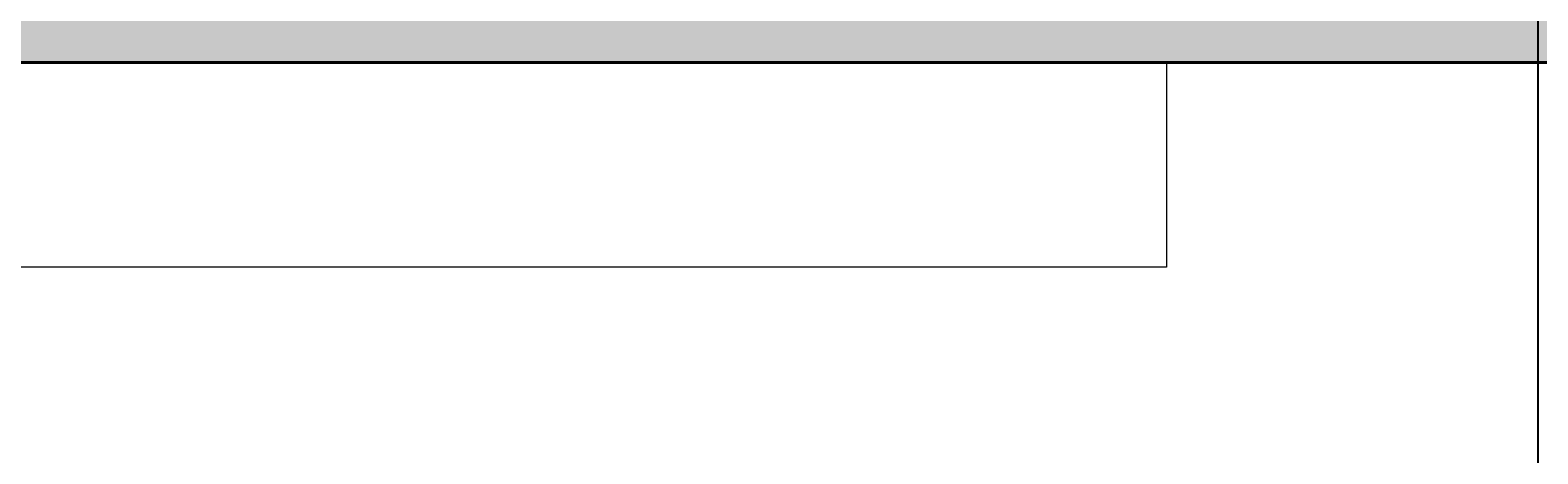
# Model space of a CAD drawing. Units: inches. Extents: x 1998 to 2588, y 1139 to 1977.
# Tile 92 of 134: x 2453 to 2498, y 1465 to 1477. Entities that reach past the tile are written whole.
import ezdxf

# ---------------------------------------------------------------- set-up
doc = ezdxf.new("R2010")
doc.units = ezdxf.units.IN
for name, color, linetype, lineweight in [('A-ANNO-DIMS', 2, 'Continuous', 18), ('A-WALL-PATT', 252, 'Continuous', 13), ('FUR', 21, 'Continuous', 18), ('WALL', 200, 'Continuous', 35)]:
    doc.layers.add(name, color=color, linetype=linetype, lineweight=lineweight)
doc.styles.get("Standard").update_dxf_attribs({"font": 'arial.ttf'})
doc.dimstyles.get("Standard").update_dxf_attribs({"dimtxt": 0.18, "dimasz": 0.18, "dimexe": 0.18, "dimexo": 0.0625, "dimgap": 0.09, "dimtad": 0, "dimtih": 1, "dimtoh": 1, "dimdec": 4, "dimzin": 0, "dimdsep": 46, "dimtxsty": 'Standard', "dimcen": 0.09, "dimadec": 0, "dimazin": 0, "dimtfac": 1, "dimtdec": 4, "dimtofl": 0, "dimtmove": 0, "dimatfit": 3, "dimfxl": 1, "dimtolj": 1, "dimtzin": 0, "dimarcsym": 0})

# ---------------------------------------------------------------- blocks, each defined once
blk = doc.blocks.new('CONSOLE-WALL')
blk.add_lwpolyline([(0, 6.123), (71.98, 6.123), (71.98, 0), (0, 0)], close=True)
blk = doc.blocks.new('*D23')
at = {"layer": 'A-ANNO-DIMS', "color": 0, "lineweight": -2, "transparency": 16777216}
for p, q in [((2549.179, 1476.17), (2549.179, 1138.602)), ((2059.473, 1413.17), (2059.473, 1138.602)), ((2059.653, 1138.782), (2303.928, 1138.782)), ((2548.999, 1138.782), (2304.723, 1138.782))]:
    blk.add_line(p, q, dxfattribs=at)
at = {"layer": 'A-ANNO-DIMS', "color": 0, "transparency": 16777216}
for points in [[(2059.653, 1138.812), (2059.653, 1138.752), (2059.473, 1138.782)], [(2548.999, 1138.812), (2548.999, 1138.752), (2549.179, 1138.782)]]:
    blk.add_solid(points, dxfattribs=at)
at = {"layer": 'Defpoints', "color": 0, "transparency": 16777216}
for p in [(2549.179, 1476.232), (2059.473, 1413.232), (2549.179, 1138.782)]:
    blk.add_point(p, dxfattribs=at)
at = {"layer": 'A-ANNO-DIMS', "color": 0, "transparency": 16777216, "insert": (2304.326, 1138.782), "char_height": 0.18, "attachment_point": 5}
blk.add_mtext('\\A1;489.7', dxfattribs=at)
blk = doc.blocks.new('*D24')
at = {"layer": 'A-ANNO-DIMS', "color": 0, "lineweight": -2, "transparency": 16777216}
for p, q in [((2398.535, 1911.232), (2588.309, 1911.232)), ((2588.129, 1911.052), (2588.129, 1570.164)), ((2588.129, 1228.912), (2588.129, 1569.8)), ((2527.535, 1228.732), (2588.309, 1228.732))]:
    blk.add_line(p, q, dxfattribs=at)
at = {"layer": 'A-ANNO-DIMS', "color": 0, "transparency": 16777216}
for points in [[(2588.099, 1911.052), (2588.159, 1911.052), (2588.129, 1911.232)], [(2588.099, 1228.912), (2588.159, 1228.912), (2588.129, 1228.732)]]:
    blk.add_solid(points, dxfattribs=at)
at = {"layer": 'Defpoints', "color": 0, "transparency": 16777216}
for p in [(2398.473, 1911.232), (2588.129, 1911.232), (2527.473, 1228.732)]:
    blk.add_point(p, dxfattribs=at)
at = {"layer": 'A-ANNO-DIMS', "color": 0, "transparency": 16777216, "insert": (2588.129, 1569.982), "char_height": 0.18, "attachment_point": 5}
blk.add_mtext('\\A1;682.5', dxfattribs=at)
blk = doc.blocks.new('*D33')
at = {"layer": 'A-ANNO-DIMS', "color": 0, "lineweight": -2, "transparency": 16777216}
for p, q in [((2407.973, 1480.67), (2407.973, 1138.602)), ((2498.179, 1480.67), (2498.179, 1138.602)), ((2408.153, 1138.782), (2452.753, 1138.782)), ((2497.999, 1138.782), (2453.399, 1138.782))]:
    blk.add_line(p, q, dxfattribs=at)
at = {"layer": 'A-ANNO-DIMS', "color": 0, "transparency": 16777216}
for points in [[(2408.153, 1138.812), (2408.153, 1138.752), (2407.973, 1138.782)], [(2497.999, 1138.812), (2497.999, 1138.752), (2498.179, 1138.782)]]:
    blk.add_solid(points, dxfattribs=at)
at = {"layer": 'Defpoints', "color": 0, "transparency": 16777216}
for p in [(2407.973, 1480.732), (2498.179, 1480.732), (2498.179, 1138.782)]:
    blk.add_point(p, dxfattribs=at)
at = {"layer": 'A-ANNO-DIMS', "color": 0, "transparency": 16777216, "insert": (2453.076, 1138.782), "char_height": 0.18, "attachment_point": 5}
blk.add_mtext('\\A1;90.2', dxfattribs=at)

msp = doc.modelspace()

# ---------------------------------------------------------------- hatches: boundary and pattern name
at = {"layer": 'A-WALL-PATT'}
h = msp.add_hatch(color=256, dxfattribs=at)
h.dxf.hatch_style = 1
h.paths.add_polyline_path([(2527.4729, 1362.2324), (2510.9729, 1362.2324), (2510.9729, 1357.7324), (2518.4729, 1357.7324), (2518.4729, 1237.7324), (2503.1458, 1237.7324), (2503.1458, 1228.7324), (2527.4729, 1228.7324)])
h.paths.add_polyline_path([(2490.5682, 1362.2324), (2398.4729, 1362.2324), (2398.4729, 1357.7324), (2490.5682, 1357.7324)])
h.paths.add_polyline_path([(2224.9729, 1264.7324), (2222.9729, 1264.7324), (2222.9729, 1232.4125), (2341.4729, 1232.4125), (2341.4729, 1234.4125), (2224.9729, 1234.4125)])
h.paths.add_polyline_path([(2334.5332, 1273.7324), (2264.7638, 1273.7324), (2264.7638, 1269.5611, -0.043659), (2264.3413, 1264.7324), (2334.5332, 1264.7324)])
h.paths.add_polyline_path([(2236.9551, 1273.7324), (2234.4125, 1273.7324), (2234.4125, 1264.7324), (2236.9551, 1264.7324), (2236.9551, 1269.5611)])
h.paths.add_polyline_path([(2222.9729, 1293.2324), (2096.9729, 1293.2324), (2096.9729, 1345.0966), (2087.9729, 1345.0966), (2087.9729, 1284.2324), (2222.9729, 1284.2324), (2222.9729, 1285.137)])
h.paths.add_polyline_path([(2096.9729, 1458.7927), (2087.9729, 1458.7927), (2087.9729, 1417.7324), (2087.9729, 1413.2324), (2096.9729, 1413.2324), (2096.9729, 1417.7324)])
h.paths.add_polyline_path([(2096.9729, 1413.2324), (2087.9729, 1413.2324), (2087.9729, 1365.5012), (2096.9729, 1365.5012), (2096.9729, 1369.3358)])
h.paths.add_polyline_path([(2186.2943, 1417.7324), (2138.6074, 1417.7324), (2096.9729, 1417.7324), (2096.9729, 1413.2324), (2138.6074, 1413.2324), (2186.2943, 1413.2324)])
h.paths.add_polyline_path([(2181.4729, 1465.7324), (2176.9729, 1465.7324), (2176.9729, 1451.6434), (2181.4729, 1451.6434)])
h.paths.add_polyline_path([(2181.4729, 1422.1664), (2176.9729, 1422.1664), (2176.9729, 1417.7324), (2181.4729, 1417.7324)])
h.paths.add_polyline_path([(2063.9729, 1465.7324), (2087.9729, 1465.7324), (2087.9729, 1470.2324), (2059.4729, 1470.2324), (2059.4729, 1413.2324), (2087.9729, 1413.2324), (2087.9729, 1417.7324), (2063.9729, 1417.7324)])
h.paths.add_polyline_path([(2181.4729, 1755.2324), (2176.9729, 1755.2324), (2176.9729, 1748.6798), (2177.0513, 1748.6798), (2181.4729, 1748.6798)])
h.paths.add_polyline_path([(2227.4729, 1707.2324), (2220.4647, 1707.2324), (2220.4647, 1702.7324), (2222.9729, 1702.7324), (2222.9729, 1604.637), (2227.4729, 1604.637)])
h.paths.add_polyline_path([(2114.9729, 1702.7324), (2105.9729, 1702.7324), (2105.9729, 1628.4781, -0.0318759), (2110.1012, 1628.7416), (2114.9729, 1628.7416)])
h.paths.add_polyline_path([(2345.9729, 1739.3278), (2341.4729, 1739.3278), (2341.4729, 1647.5211), (2345.9729, 1647.5211)])
h.paths.add_polyline_path([(2350.6273, 1641.2324), (2345.9729, 1641.2324), (2345.9729, 1636.7324), (2350.6273, 1636.7324), (2350.6273, 1639.8729)])
h.paths.add_polyline_path([(2501.9729, 1641.2324), (2407.9729, 1641.2324), (2392.5005, 1641.2324), (2392.5005, 1639.8729), (2392.5005, 1636.7324), (2501.9729, 1636.7324)])
h.paths.add_polyline_path([(2510.9729, 1755.2324), (2501.9729, 1755.2324), (2501.9729, 1641.2324), (2510.9729, 1641.2324)])
h.paths.add_polyline_path([(2549.1786, 1641.2324), (2522.3775, 1641.2324), (2522.3775, 1636.7324), (2540.1786, 1636.7324), (2540.1786, 1480.7324), (2522.3775, 1480.7324), (2522.3775, 1476.2324), (2549.1786, 1476.2324)])
h.paths.add_polyline_path([(2498.1786, 1594.7324), (2407.9729, 1594.7324), (2407.9729, 1585.7324), (2416.9729, 1585.7324), (2489.1786, 1585.7324), (2489.1786, 1531.7324), (2416.9729, 1531.7324), (2407.9729, 1531.7324), (2407.9729, 1522.7324), (2498.1786, 1522.7324)])
h.paths.add_polyline_path([(2351.6437, 1480.7324), (2345.9729, 1480.7324), (2345.9729, 1476.2324), (2351.6437, 1476.2324), (2351.6437, 1477.5919)])
h.paths.add_polyline_path([(2501.9729, 1480.7324), (2498.1786, 1480.7324), (2407.9729, 1480.7324), (2393.5168, 1480.7324), (2393.5168, 1477.5919), (2393.5168, 1476.2324), (2501.9729, 1476.2324)])

# ---------------------------------------------------------------- linework, layer by layer
at = {"layer": 'WALL'}
for p, q in [((2392.6008, 1476.2324), (2501.9729, 1476.2324)), ((2501.9729, 1476.2324), (2407.9729, 1476.2324))]:
    msp.add_line(p, q, dxfattribs=at)

# ---------------------------------------------------------------- block references
at = {"layer": 'FUR'}
msp.add_blockref('CONSOLE-WALL', (2415.1012, 1470.109), dxfattribs=at)

# ---------------------------------------------------------------- dimensions: what is measured, and where the dimension line sits
at = {"layer": 'A-ANNO-DIMS'}
dim = msp.add_linear_dim(base=(2588.1286, 1911.2324), p1=(2527.4729, 1228.7324), p2=(2398.4729, 1911.2324), angle=90, dimstyle='Standard', override={"dimdec": 1, "dimlfac": 1, "dimrnd": 0, "dimzin": 0, "dimdsep": 46, "dimlunit": 2}, dxfattribs=at)
dim.commit()
dim.dimension.update_dxf_attribs({"geometry": '*D24', "text_midpoint": (2588.1286, 1569.9824)})
for base, p1, p2, picture, middle in [((2498.1786, 1138.7824), (2407.9729, 1480.7324), (2498.1786, 1480.7324), '*D33', (2453.0757, 1138.7824)), ((2549.1786, 1138.7824), (2059.4729, 1413.2324), (2549.1786, 1476.2324), '*D23', (2304.3257, 1138.7824))]:
    dim = msp.add_linear_dim(base=base, p1=p1, p2=p2, dimstyle='Standard', override={"dimdec": 1, "dimlfac": 1, "dimrnd": 0, "dimzin": 0, "dimdsep": 46, "dimlunit": 2}, dxfattribs=at)
    dim.commit()
    dim.dimension.update_dxf_attribs({"geometry": picture, "text_midpoint": middle})

doc.saveas('drawing.dxf')
